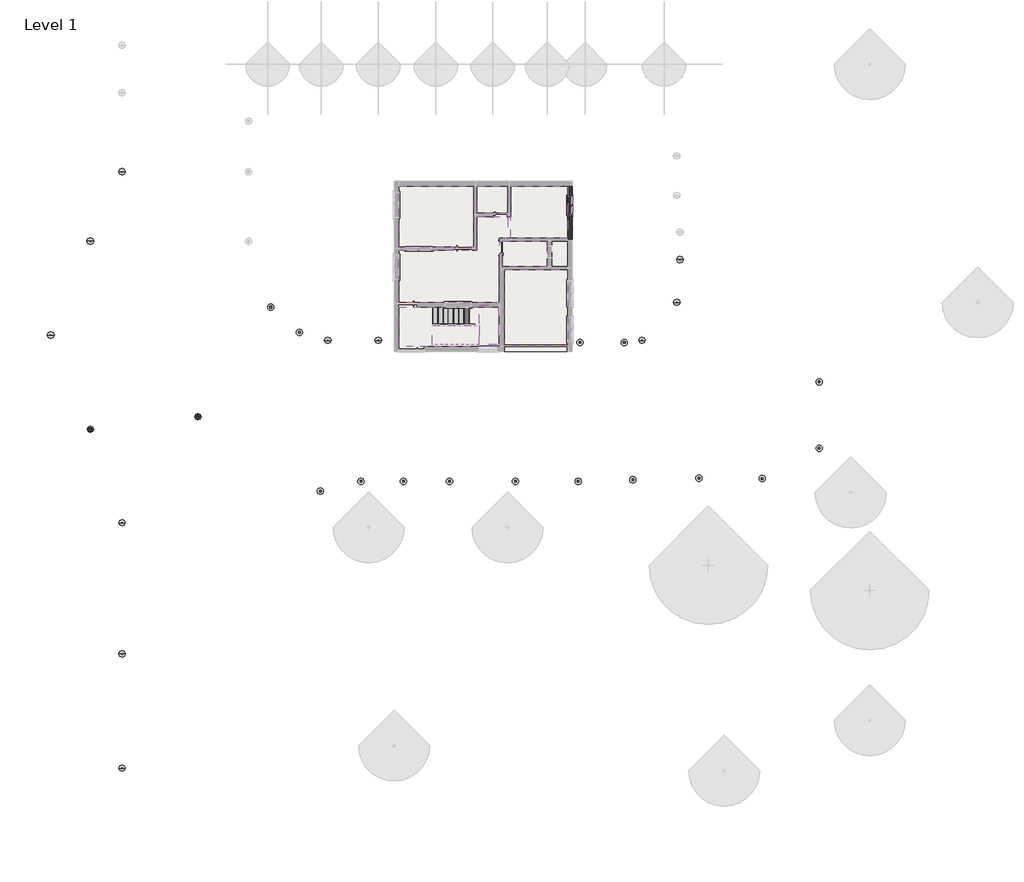
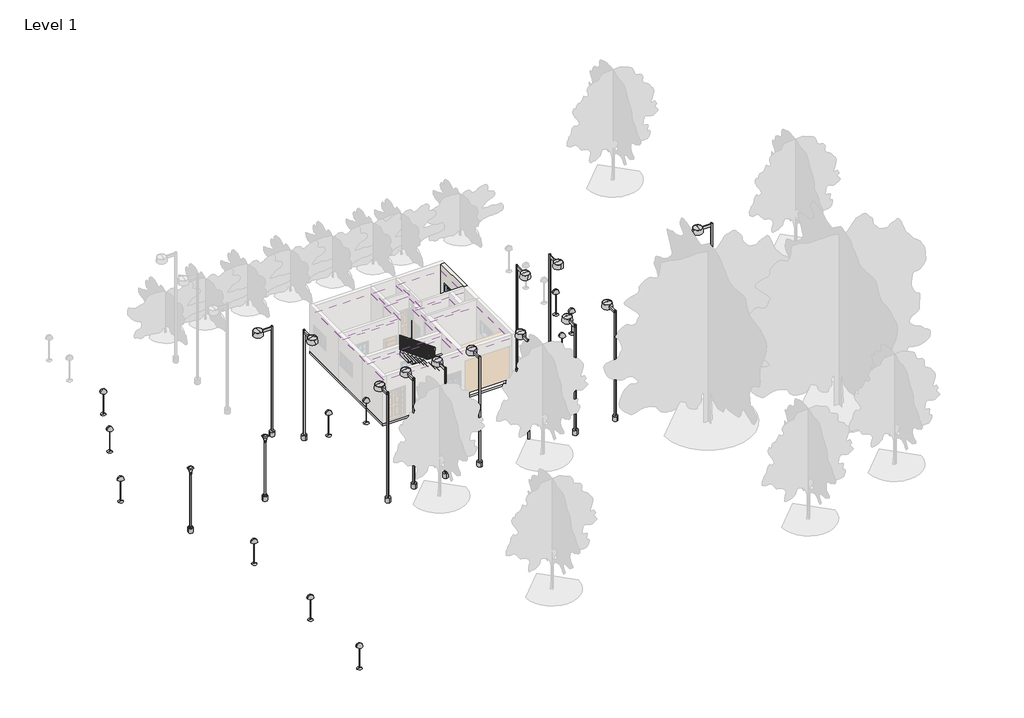
# One storey, part 2 of 3: 28 light fixtures, 7 coverings, 2 slabs, 2 stair flights, 1 railing, 1 wall, 1 window.
"""IFC4 building model written with IfcOpenShell, lengths in millimetres."""

from ifc_helpers import new_model, si_unit, frame, origin, place, context, project, spatial, polyline, outline, extrude, faceted_brep, transform, mapped, element, save
from components import m_floor_lamp_hemispheric_60w_120v_4a08ccbb, m_street_light_antique_400w_halogen_120v_ac89fb25, m_street_light_standard_250w_halogen_480v_204dbcbb, non_monolithic_landing_adbeca5e, stair_flight_50mm_tread_13mm_riser_with_nosing_6f61a695, stair_flight_50mm_tread_13mm_riser_with_nosing_ea10009b, m_window_casement_double_awning_double_3_6fa9dbfe

model = new_model("IFC4")

# Units and contexts
model_context = context("Model", 3, world=origin())
ifc_project = project(units=[si_unit("LENGTHUNIT", "METRE", prefix="MILLI")], contexts=[model_context])

# Site, building, storey
site = spatial("IfcSite", under=ifc_project)
building = spatial("IfcBuilding", under=site)
storey = spatial("IfcBuildingStorey", under=building, Name="Level 1", Elevation=0.0)

# Coverings
placement = place(None, origin())
element("IfcCovering", 1, ObjectType="Plain", at=placement, inside=storey, context=model_context, shape_type="SweptSolid", body=[
    extrude(outline(polyline([(-7823.0282945, 467.5578397), (-11429.8282945, 467.5578397), (-11429.8282945, 3413.9578397), (-7823.0282945, 3413.9578397), (-7823.0282945, 467.5578397)])), frame((0.0, 0.0, 2743.2), z_axis=(0.0, 0.0, 1.0), x_axis=(1.0, 0.0, 0.0)), (0.0, 0.0, 1.0), 57.0),
])
element("IfcCovering", 2, ObjectType="Plain", at=placement, inside=storey, context=model_context, shape_type="SweptSolid", body=[
    extrude(outline(polyline([(-7670.6282945, 2093.1578397), (-7670.6282945, 3413.9578397), (-6197.4282945, 3413.9578397), (-6197.4282945, 2093.1578397), (-7670.6282945, 2093.1578397)])), frame((0.0, 0.0, 2743.2), z_axis=(0.0, 0.0, 1.0), x_axis=(1.0, 0.0, 0.0)), (0.0, 0.0, 1.0), 57.0),
])
element("IfcCovering", 3, ObjectType="Plain", at=placement, inside=storey, context=model_context, shape_type="SweptSolid", body=[
    extrude(outline(polyline([(-11429.8282945, -2199.4421603), (-11429.8282945, 315.1578397), (-7670.6282945, 315.1578397), (-7670.6282945, 1940.7578397), (-6197.4282945, 1940.7578397), (-6197.4282945, 899.3578397), (-6603.8282945, 899.3578397), (-6603.8282945, -548.4421603), (-6603.8282945, -2199.4421603), (-11429.8282945, -2199.4421603)])), frame((0.0, 0.0, 2743.2), z_axis=(0.0, 0.0, 1.0), x_axis=(1.0, 0.0, 0.0)), (0.0, 0.0, 1.0), 57.0),
])
element("IfcCovering", 4, ObjectType="Plain", at=placement, inside=storey, context=model_context, shape_type="SweptSolid", body=[
    extrude(outline(polyline([(-6045.0282945, 899.3578397), (-6045.0282945, 3413.9578397), (-3301.8282945, 3413.9578397), (-3301.8282945, 899.3578397), (-6045.0282945, 899.3578397)])), frame((0.0, 0.0, 2743.2), z_axis=(0.0, 0.0, 1.0), x_axis=(1.0, 0.0, 0.0)), (0.0, 0.0, 1.0), 57.0),
])
element("IfcCovering", 5, ObjectType="Plain", at=placement, inside=storey, context=model_context, shape_type="SweptSolid", body=[
    extrude(outline(polyline([(-6451.4282945, 746.9578397), (-4292.4282945, 746.9578397), (-4292.4282945, -472.2421603), (-6451.4282945, -472.2421603), (-6451.4282945, 746.9578397)])), frame((0.0, 0.0, 2743.2), z_axis=(0.0, 0.0, 1.0), x_axis=(1.0, 0.0, 0.0)), (0.0, 0.0, 1.0), 57.0),
])
element("IfcCovering", 6, ObjectType="Plain", at=placement, inside=storey, context=model_context, shape_type="SweptSolid", body=[
    extrude(outline(polyline([(-6349.8282945, -624.6421603), (-3301.8282945, -624.6421603), (-3301.8282945, -4333.0421603), (-6349.8282945, -4333.0421603), (-6349.8282945, -624.6421603)])), frame((0.0, 0.0, 2743.2), z_axis=(0.0, 0.0, 1.0), x_axis=(1.0, 0.0, 0.0)), (0.0, 0.0, 1.0), 57.0),
])
element("IfcCovering", 7, ObjectType="Plain", at=placement, inside=storey, context=model_context, shape_type="SweptSolid", body=[
    extrude(outline(polyline([(-11429.8282945, -4333.0421603), (-11429.8282945, -2428.0421603), (-6603.8282945, -2428.0421603), (-6603.8282945, -4333.0421603), (-11429.8282945, -4333.0421603)])), frame((0.0, 0.0, 2743.2), z_axis=(0.0, 0.0, 1.0), x_axis=(1.0, 0.0, 0.0)), (0.0, 0.0, 1.0), 57.0),
])

# Light fixtures
m_floor_lamp_hemispheric_60w_120v_shape = m_floor_lamp_hemispheric_60w_120v_4a08ccbb(model_context)
element("IfcLightFixture", 8, ObjectType="M_Floor Lamp - Hemispheric : 60W - 120V", at=placement, inside=storey, context=model_context, shape_type="MappedRepresentation", body=[
    mapped(m_floor_lamp_hemispheric_60w_120v_shape, transform((-24764.8282945, 4099.7578397, 0.0), x_axis=(1.0, 0.0, 0.0), y_axis=(0.0, 1.0, 0.0), z_axis=(0.0, 0.0, 1.0))),
])
element("IfcLightFixture", 9, ObjectType="M_Floor Lamp - Hemispheric : 60W - 120V", at=placement, inside=storey, context=model_context, shape_type="MappedRepresentation", body=[
    mapped(m_floor_lamp_hemispheric_60w_120v_shape, transform((-26288.8282945, 746.9578397, 0.0), x_axis=(1.0, 0.0, 0.0), y_axis=(0.0, 1.0, 0.0), z_axis=(0.0, 0.0, 1.0))),
])
element("IfcLightFixture", 10, ObjectType="M_Floor Lamp - Hemispheric : 60W - 120V", at=placement, inside=storey, context=model_context, shape_type="MappedRepresentation", body=[
    mapped(m_floor_lamp_hemispheric_60w_120v_shape, transform((-28199.496103, -3776.7092743, 0.0), x_axis=(1.0, 0.0, 0.0), y_axis=(0.0, 1.0, 0.0), z_axis=(0.0, 0.0, 1.0))),
])
element("IfcLightFixture", 11, ObjectType="M_Floor Lamp - Hemispheric : 60W - 120V", at=placement, inside=storey, context=model_context, shape_type="MappedRepresentation", body=[
    mapped(m_floor_lamp_hemispheric_60w_120v_shape, transform((-24764.8282945, -12820.2421603, 0.0), x_axis=(1.0, 0.0, 0.0), y_axis=(0.0, 1.0, 0.0), z_axis=(0.0, 0.0, 1.0))),
])
element("IfcLightFixture", 12, ObjectType="M_Floor Lamp - Hemispheric : 60W - 120V", at=placement, inside=storey, context=model_context, shape_type="MappedRepresentation", body=[
    mapped(m_floor_lamp_hemispheric_60w_120v_shape, transform((-24764.8282945, -19145.2421603, 0.0), x_axis=(1.0, 0.0, 0.0), y_axis=(0.0, 1.0, 0.0), z_axis=(0.0, 0.0, 1.0))),
])
element("IfcLightFixture", 13, ObjectType="M_Floor Lamp - Hemispheric : 60W - 120V", at=placement, inside=storey, context=model_context, shape_type="MappedRepresentation", body=[
    mapped(m_floor_lamp_hemispheric_60w_120v_shape, transform((-24764.8282945, -24645.2421603, 0.0), x_axis=(1.0, 0.0, 0.0), y_axis=(0.0, 1.0, 0.0), z_axis=(0.0, 0.0, 1.0))),
])
element("IfcLightFixture", 14, ObjectType="M_Floor Lamp - Hemispheric : 60W - 120V", at=placement, inside=storey, context=model_context, shape_type="MappedRepresentation", body=[
    mapped(m_floor_lamp_hemispheric_60w_120v_shape, transform((2108.3717055, -142.0421603, 0.0), x_axis=(1.0, 0.0, 0.0), y_axis=(0.0, 1.0, 0.0), z_axis=(0.0, 0.0, 1.0))),
])
element("IfcLightFixture", 15, ObjectType="M_Floor Lamp - Hemispheric : 60W - 120V", at=placement, inside=storey, context=model_context, shape_type="MappedRepresentation", body=[
    mapped(m_floor_lamp_hemispheric_60w_120v_shape, transform((1955.9717055, -2199.4421603, 0.0), x_axis=(1.0, 0.0, 0.0), y_axis=(0.0, 1.0, 0.0), z_axis=(0.0, 0.0, 1.0))),
])
element("IfcLightFixture", 16, ObjectType="M_Floor Lamp - Hemispheric : 60W - 120V", at=placement, inside=storey, context=model_context, shape_type="MappedRepresentation", body=[
    mapped(m_floor_lamp_hemispheric_60w_120v_shape, transform((279.5717055, -4028.2421603, 0.0), x_axis=(1.0, 0.0, 0.0), y_axis=(0.0, 1.0, 0.0), z_axis=(0.0, 0.0, 1.0))),
])
element("IfcLightFixture", 17, ObjectType="M_Floor Lamp - Hemispheric : 60W - 120V", at=placement, inside=storey, context=model_context, shape_type="MappedRepresentation", body=[
    mapped(m_floor_lamp_hemispheric_60w_120v_shape, transform((-12420.4282945, -4028.2421603, 0.0), x_axis=(1.0, 0.0, 0.0), y_axis=(0.0, 1.0, 0.0), z_axis=(0.0, 0.0, 1.0))),
])
element("IfcLightFixture", 18, ObjectType="M_Floor Lamp - Hemispheric : 60W - 120V", at=placement, inside=storey, context=model_context, shape_type="MappedRepresentation", body=[
    mapped(m_floor_lamp_hemispheric_60w_120v_shape, transform((-14858.8282945, -4028.2421603, 0.0), x_axis=(1.0, 0.0, 0.0), y_axis=(0.0, 1.0, 0.0), z_axis=(0.0, 0.0, 1.0))),
])
m_street_light_antique_400w_halogen_120v_shape = m_street_light_antique_400w_halogen_120v_ac89fb25(model_context)
element("IfcLightFixture", 19, ObjectType="M_Street Light - Antique : 400W Halogen - 120V", at=placement, inside=storey, context=model_context, shape_type="MappedRepresentation", body=[
    mapped(m_street_light_antique_400w_halogen_120v_shape, transform((-21107.2282945, -7711.2421603, 0.0), x_axis=(1.0, 0.0, 0.0), y_axis=(0.0, 1.0, 0.0), z_axis=(0.0, 0.0, 1.0))),
])
element("IfcLightFixture", 20, ObjectType="M_Street Light - Antique : 400W Halogen - 120V", at=placement, inside=storey, context=model_context, shape_type="MappedRepresentation", body=[
    mapped(m_street_light_antique_400w_halogen_120v_shape, transform((-26288.8282945, -8320.8421603, 0.0), x_axis=(1.0, 0.0, 0.0), y_axis=(0.0, 1.0, 0.0), z_axis=(0.0, 0.0, 1.0))),
])
m_street_light_standard_250w_halogen_480v_shape = m_street_light_standard_250w_halogen_480v_204dbcbb(model_context)
element("IfcLightFixture", 21, ObjectType="M_Street Light - Standard : 250W Halogen - 480V", at=placement, inside=storey, context=model_context, shape_type="MappedRepresentation", body=[
    mapped(m_street_light_standard_250w_halogen_480v_shape, transform((-15213.0614004, -11296.4871366, 0.0), x_axis=(0.0, -1.0, 0.0), y_axis=(1.0, 0.0, 0.0), z_axis=(0.0, 0.0, 1.0))),
])
element("IfcLightFixture", 22, ObjectType="M_Street Light - Standard : 250W Halogen - 480V", at=placement, inside=storey, context=model_context, shape_type="MappedRepresentation", body=[
    mapped(m_street_light_standard_250w_halogen_480v_shape, transform((-13256.1020795, -10825.1754443, 0.0), x_axis=(0.0, -1.0, 0.0), y_axis=(1.0, 0.0, 0.0), z_axis=(0.0, 0.0, 1.0))),
])
element("IfcLightFixture", 23, ObjectType="M_Street Light - Standard : 250W Halogen - 480V", at=placement, inside=storey, context=model_context, shape_type="MappedRepresentation", body=[
    mapped(m_street_light_standard_250w_halogen_480v_shape, transform((-11210.6990221, -10825.1754443, 0.0), x_axis=(0.0, -1.0, 0.0), y_axis=(1.0, 0.0, 0.0), z_axis=(0.0, 0.0, 1.0))),
])
element("IfcLightFixture", 24, ObjectType="M_Street Light - Standard : 250W Halogen - 480V", at=placement, inside=storey, context=model_context, shape_type="MappedRepresentation", body=[
    mapped(m_street_light_standard_250w_halogen_480v_shape, transform((-8991.4282945, -10825.1754443, 0.0), x_axis=(0.0, -1.0, 0.0), y_axis=(1.0, 0.0, 0.0), z_axis=(0.0, 0.0, 1.0))),
])
element("IfcLightFixture", 25, ObjectType="M_Street Light - Standard : 250W Halogen - 480V", at=placement, inside=storey, context=model_context, shape_type="MappedRepresentation", body=[
    mapped(m_street_light_standard_250w_halogen_480v_shape, transform((-5816.409264, -10825.1754443, 0.0), x_axis=(0.0, -1.0, 0.0), y_axis=(1.0, 0.0, 0.0), z_axis=(0.0, 0.0, 1.0))),
])
element("IfcLightFixture", 26, ObjectType="M_Street Light - Standard : 250W Halogen - 480V", at=placement, inside=storey, context=model_context, shape_type="MappedRepresentation", body=[
    mapped(m_street_light_standard_250w_halogen_480v_shape, transform((-2793.8282945, -10825.1754443, 0.0), x_axis=(0.0, -1.0, 0.0), y_axis=(1.0, 0.0, 0.0), z_axis=(0.0, 0.0, 1.0))),
])
element("IfcLightFixture", 27, ObjectType="M_Street Light - Standard : 250W Halogen - 480V", at=placement, inside=storey, context=model_context, shape_type="MappedRepresentation", body=[
    mapped(m_street_light_standard_250w_halogen_480v_shape, transform((-160.8463909, -10748.9754443, 0.0), x_axis=(0.0, -1.0, 0.0), y_axis=(1.0, 0.0, 0.0), z_axis=(0.0, 0.0, 1.0))),
])
element("IfcLightFixture", 28, ObjectType="M_Street Light - Standard : 250W Halogen - 480V", at=placement, inside=storey, context=model_context, shape_type="MappedRepresentation", body=[
    mapped(m_street_light_standard_250w_halogen_480v_shape, transform((3022.7717055, -10672.7754443, 0.0), x_axis=(0.0, -1.0, 0.0), y_axis=(1.0, 0.0, 0.0), z_axis=(0.0, 0.0, 1.0))),
])
element("IfcLightFixture", 29, ObjectType="M_Street Light - Standard : 250W Halogen - 480V", at=placement, inside=storey, context=model_context, shape_type="MappedRepresentation", body=[
    mapped(m_street_light_standard_250w_halogen_480v_shape, transform((8813.9717055, -6034.8421603, 0.0), x_axis=(1.0, 0.0, 0.0), y_axis=(0.0, 1.0, 0.0), z_axis=(0.0, 0.0, 1.0))),
])
element("IfcLightFixture", 30, ObjectType="M_Street Light - Standard : 250W Halogen - 480V", at=placement, inside=storey, context=model_context, shape_type="MappedRepresentation", body=[
    mapped(m_street_light_standard_250w_halogen_480v_shape, transform((8813.9717055, -9235.2421603, 0.0), x_axis=(1.0, 0.0, 0.0), y_axis=(0.0, 1.0, 0.0), z_axis=(0.0, 0.0, 1.0))),
])
element("IfcLightFixture", 31, ObjectType="M_Street Light - Standard : 250W Halogen - 480V", at=placement, inside=storey, context=model_context, shape_type="MappedRepresentation", body=[
    mapped(m_street_light_standard_250w_halogen_480v_shape, transform((6070.7717055, -10690.9806356, 0.0), x_axis=(0.0, -1.0, 0.0), y_axis=(1.0, 0.0, 0.0), z_axis=(0.0, 0.0, 1.0))),
])
element("IfcLightFixture", 32, ObjectType="M_Street Light - Standard : 400W Halogen - 120V", at=placement, inside=storey, context=model_context, shape_type="MappedRepresentation", body=[
    mapped(m_street_light_standard_250w_halogen_480v_shape, transform((-17602.0282945, -2428.0421603, 0.0), x_axis=(1.0, 0.0, 0.0), y_axis=(0.0, 1.0, 0.0), z_axis=(0.0, 0.0, 1.0))),
])
element("IfcLightFixture", 33, ObjectType="M_Street Light - Standard : 400W Halogen - 120V", at=placement, inside=storey, context=model_context, shape_type="MappedRepresentation", body=[
    mapped(m_street_light_standard_250w_halogen_480v_shape, transform((-16221.6329612, -3647.2421603, 0.0), x_axis=(0.0, 1.0, 0.0), y_axis=(-1.0, 0.0, 0.0), z_axis=(0.0, 0.0, 1.0))),
])
element("IfcLightFixture", 34, ObjectType="M_Street Light - Standard : 400W Halogen - 120V", at=placement, inside=storey, context=model_context, shape_type="MappedRepresentation", body=[
    mapped(m_street_light_standard_250w_halogen_480v_shape, transform((-575.2329612, -4129.8421603, 0.0), x_axis=(0.0, 1.0, 0.0), y_axis=(-1.0, 0.0, 0.0), z_axis=(0.0, 0.0, 1.0))),
])
element("IfcLightFixture", 35, ObjectType="M_Street Light - Standard : 400W Halogen - 120V", at=placement, inside=storey, context=model_context, shape_type="MappedRepresentation", body=[
    mapped(m_street_light_standard_250w_halogen_480v_shape, transform((-2708.8329612, -4129.8421603, 0.0), x_axis=(0.0, 1.0, 0.0), y_axis=(-1.0, 0.0, 0.0), z_axis=(0.0, 0.0, 1.0))),
])

# Railing
element("IfcRailing", 36, ObjectType="1100mm", at=placement, inside=storey, context=model_context, shape_type="SolidModel", body=[
    faceted_brep([(-9804.2282945, -3247.1921603, 1277.8), (-9804.2282945, -3247.1921603, 1216.4443678), (-9804.2282945, -3297.1921603, 1216.4443678), (-9804.2282945, -3297.1921603, 1277.8), (-7604.2282945, -3247.1921603, 2842.44), (-7604.2282945, -3297.1921603, 2842.44), (-7604.2282945, -3297.1921603, 2781.0843678), (-7604.2282945, -3247.1921603, 2781.0843678)], [[[0, 1, 2, 3]], [[4, 5, 6, 7]], [[1, 0, 4, 7]], [[2, 1, 7, 6]], [[3, 2, 6, 5]], [[0, 3, 5, 4]]]),
    faceted_brep([(-7554.2282945, -3323.3921603, 3055.8), (-7604.2282945, -3323.3921603, 3030.0043678), (-7604.2282945, -3273.3921603, 3030.0043678), (-7554.2282945, -3273.3921603, 3055.8), (-9804.2282945, -3323.3921603, 4656.0), (-9804.2282945, -3273.3921603, 4656.0), (-9804.2282945, -3273.3921603, 4594.6443678), (-9804.2282945, -3323.3921603, 4594.6443678)], [[[0, 1, 2, 3]], [[4, 5, 6, 7]], [[1, 0, 4, 7]], [[2, 1, 7, 6]], [[3, 2, 6, 5]], [[0, 3, 5, 4]]]),
    faceted_brep([(-7554.2282945, -3247.1921603, 2878.0), (-7554.2282945, -3247.1921603, 2828.0), (-7604.2282945, -3247.1921603, 2828.0), (-7604.2282945, -3247.1921603, 2878.0), (-7554.2282945, -3273.3921603, 2878.0), (-7604.2282945, -3273.3921603, 2878.0), (-7604.2282945, -3323.3921603, 2828.0), (-7554.2282945, -3323.3921603, 2828.0)], [[[0, 1, 2, 3]], [[4, 5, 6, 7]], [[1, 0, 4, 7]], [[2, 1, 7, 6]], [[3, 2, 6, 5]], [[0, 3, 5, 4]]]),
    faceted_brep([(-7554.2282945, -3273.3921603, 2878.0), (-7554.2282945, -3323.3921603, 2828.0), (-7604.2282945, -3323.3921603, 2828.0), (-7604.2282945, -3273.3921603, 2878.0), (-7554.2282945, -3273.3921603, 3055.8), (-7604.2282945, -3273.3921603, 3030.0043678), (-7604.2282945, -3323.3921603, 3030.0043678), (-7554.2282945, -3323.3921603, 3055.8)], [[[0, 1, 2, 3]], [[4, 5, 6, 7]], [[1, 0, 4, 7]], [[2, 1, 7, 6]], [[3, 2, 6, 5]], [[0, 3, 5, 4]]]),
    extrude(outline(polyline([(3590.5281609, -9754.2282945), (4559.0843678, -9754.2282945), (4576.8643678, -9779.2282945), (3608.3081609, -9779.2282945), (3590.5281609, -9754.2282945)])), frame((0.0, -3310.8921603, 0.0), z_axis=(0.0, 1.0, 0.0), x_axis=(0.0, 0.0, 1.0)), (0.0, 0.0, 1.0), 25.0),
    extrude(outline(polyline([(3501.6281609, -9629.2282945), (4470.1843678, -9629.2282945), (4487.9643678, -9654.2282945), (3519.4081609, -9654.2282945), (3501.6281609, -9629.2282945)])), frame((0.0, -3310.8921603, 0.0), z_axis=(0.0, 1.0, 0.0), x_axis=(0.0, 0.0, 1.0)), (0.0, 0.0, 1.0), 25.0),
    extrude(outline(polyline([(3412.7281609, -9504.2282945), (4381.2843678, -9504.2282945), (4399.0643678, -9529.2282945), (3430.5081609, -9529.2282945), (3412.7281609, -9504.2282945)])), frame((0.0, -3310.8921603, 0.0), z_axis=(0.0, 1.0, 0.0), x_axis=(0.0, 0.0, 1.0)), (0.0, 0.0, 1.0), 25.0),
    extrude(outline(polyline([(3323.8281609, -9379.2282945), (4292.3843678, -9379.2282945), (4310.1643678, -9404.2282945), (3341.6081609, -9404.2282945), (3323.8281609, -9379.2282945)])), frame((0.0, -3310.8921603, 0.0), z_axis=(0.0, 1.0, 0.0), x_axis=(0.0, 0.0, 1.0)), (0.0, 0.0, 1.0), 25.0),
    extrude(outline(polyline([(3234.9281609, -9254.2282945), (4203.4843678, -9254.2282945), (4221.2643678, -9279.2282945), (3252.7081609, -9279.2282945), (3234.9281609, -9254.2282945)])), frame((0.0, -3310.8921603, 0.0), z_axis=(0.0, 1.0, 0.0), x_axis=(0.0, 0.0, 1.0)), (0.0, 0.0, 1.0), 25.0),
    extrude(outline(polyline([(3146.0281609, -9129.2282945), (4114.5843678, -9129.2282945), (4132.3643678, -9154.2282945), (3163.8081609, -9154.2282945), (3146.0281609, -9129.2282945)])), frame((0.0, -3310.8921603, 0.0), z_axis=(0.0, 1.0, 0.0), x_axis=(0.0, 0.0, 1.0)), (0.0, 0.0, 1.0), 25.0),
    extrude(outline(polyline([(3057.1281609, -9004.2282945), (4025.6843678, -9004.2282945), (4043.4643678, -9029.2282945), (3074.9081609, -9029.2282945), (3057.1281609, -9004.2282945)])), frame((0.0, -3310.8921603, 0.0), z_axis=(0.0, 1.0, 0.0), x_axis=(0.0, 0.0, 1.0)), (0.0, 0.0, 1.0), 25.0),
    extrude(outline(polyline([(2968.2281609, -8879.2282945), (3936.7843678, -8879.2282945), (3954.5643678, -8904.2282945), (2986.0081609, -8904.2282945), (2968.2281609, -8879.2282945)])), frame((0.0, -3310.8921603, 0.0), z_axis=(0.0, 1.0, 0.0), x_axis=(0.0, 0.0, 1.0)), (0.0, 0.0, 1.0), 25.0),
    extrude(outline(polyline([(2879.3281609, -8754.2282945), (3847.8843678, -8754.2282945), (3865.6643678, -8779.2282945), (2897.1081609, -8779.2282945), (2879.3281609, -8754.2282945)])), frame((0.0, -3310.8921603, 0.0), z_axis=(0.0, 1.0, 0.0), x_axis=(0.0, 0.0, 1.0)), (0.0, 0.0, 1.0), 25.0),
    extrude(outline(polyline([(2790.4281609, -8629.2282945), (3758.9843678, -8629.2282945), (3776.7643678, -8654.2282945), (2808.2081609, -8654.2282945), (2790.4281609, -8629.2282945)])), frame((0.0, -3310.8921603, 0.0), z_axis=(0.0, 1.0, 0.0), x_axis=(0.0, 0.0, 1.0)), (0.0, 0.0, 1.0), 25.0),
    extrude(outline(polyline([(2701.5281609, -8504.2282945), (3670.0843678, -8504.2282945), (3687.8643678, -8529.2282945), (2719.3081609, -8529.2282945), (2701.5281609, -8504.2282945)])), frame((0.0, -3310.8921603, 0.0), z_axis=(0.0, 1.0, 0.0), x_axis=(0.0, 0.0, 1.0)), (0.0, 0.0, 1.0), 25.0),
    extrude(outline(polyline([(2612.6281609, -8379.2282945), (3581.1843678, -8379.2282945), (3598.9643678, -8404.2282945), (2630.4081609, -8404.2282945), (2612.6281609, -8379.2282945)])), frame((0.0, -3310.8921603, 0.0), z_axis=(0.0, 1.0, 0.0), x_axis=(0.0, 0.0, 1.0)), (0.0, 0.0, 1.0), 25.0),
    extrude(outline(polyline([(2523.7281609, -8254.2282945), (3492.2843678, -8254.2282945), (3510.0643678, -8279.2282945), (2541.5081609, -8279.2282945), (2523.7281609, -8254.2282945)])), frame((0.0, -3310.8921603, 0.0), z_axis=(0.0, 1.0, 0.0), x_axis=(0.0, 0.0, 1.0)), (0.0, 0.0, 1.0), 25.0),
    extrude(outline(polyline([(2434.8281609, -8129.2282945), (3403.3843678, -8129.2282945), (3421.1643678, -8154.2282945), (2452.6081609, -8154.2282945), (2434.8281609, -8129.2282945)])), frame((0.0, -3310.8921603, 0.0), z_axis=(0.0, 1.0, 0.0), x_axis=(0.0, 0.0, 1.0)), (0.0, 0.0, 1.0), 25.0),
    extrude(outline(polyline([(2345.9281609, -8004.2282945), (3314.4843678, -8004.2282945), (3332.2643678, -8029.2282945), (2363.7081609, -8029.2282945), (2345.9281609, -8004.2282945)])), frame((0.0, -3310.8921603, 0.0), z_axis=(0.0, 1.0, 0.0), x_axis=(0.0, 0.0, 1.0)), (0.0, 0.0, 1.0), 25.0),
    extrude(outline(polyline([(2257.0281609, -7879.2282945), (3225.5843678, -7879.2282945), (3243.3643678, -7904.2282945), (2274.8081609, -7904.2282945), (2257.0281609, -7879.2282945)])), frame((0.0, -3310.8921603, 0.0), z_axis=(0.0, 1.0, 0.0), x_axis=(0.0, 0.0, 1.0)), (0.0, 0.0, 1.0), 25.0),
    extrude(outline(polyline([(2168.1281609, -7754.2282945), (3136.6843678, -7754.2282945), (3154.4643678, -7779.2282945), (2185.9081609, -7779.2282945), (2168.1281609, -7754.2282945)])), frame((0.0, -3310.8921603, 0.0), z_axis=(0.0, 1.0, 0.0), x_axis=(0.0, 0.0, 1.0)), (0.0, 0.0, 1.0), 25.0),
    extrude(outline(polyline([(2079.2281609, -7629.2282945), (3047.7843678, -7629.2282945), (3065.5643678, -7654.2282945), (2097.0081609, -7654.2282945), (2079.2281609, -7629.2282945)])), frame((0.0, -3310.8921603, 0.0), z_axis=(0.0, 1.0, 0.0), x_axis=(0.0, 0.0, 1.0)), (0.0, 0.0, 1.0), 25.0),
    extrude(outline(polyline([(2763.3043678, -7629.2282945), (1794.7481609, -7629.2282945), (1812.5281609, -7604.2282945), (2781.0843678, -7604.2282945), (2763.3043678, -7629.2282945)])), frame((0.0, -3284.6921603, 0.0), z_axis=(0.0, 1.0, 0.0), x_axis=(0.0, 0.0, 1.0)), (0.0, 0.0, 1.0), 25.0),
    extrude(outline(polyline([(2674.4043678, -7754.2282945), (1705.8481609, -7754.2282945), (1723.6281609, -7729.2282945), (2692.1843678, -7729.2282945), (2674.4043678, -7754.2282945)])), frame((0.0, -3284.6921603, 0.0), z_axis=(0.0, 1.0, 0.0), x_axis=(0.0, 0.0, 1.0)), (0.0, 0.0, 1.0), 25.0),
    extrude(outline(polyline([(2585.5043678, -7879.2282945), (1616.9481609, -7879.2282945), (1634.7281609, -7854.2282945), (2603.2843678, -7854.2282945), (2585.5043678, -7879.2282945)])), frame((0.0, -3284.6921603, 0.0), z_axis=(0.0, 1.0, 0.0), x_axis=(0.0, 0.0, 1.0)), (0.0, 0.0, 1.0), 25.0),
    extrude(outline(polyline([(2496.6043678, -8004.2282945), (1528.0481609, -8004.2282945), (1545.8281609, -7979.2282945), (2514.3843678, -7979.2282945), (2496.6043678, -8004.2282945)])), frame((0.0, -3284.6921603, 0.0), z_axis=(0.0, 1.0, 0.0), x_axis=(0.0, 0.0, 1.0)), (0.0, 0.0, 1.0), 25.0),
    extrude(outline(polyline([(2407.7043678, -8129.2282945), (1439.1481609, -8129.2282945), (1456.9281609, -8104.2282945), (2425.4843678, -8104.2282945), (2407.7043678, -8129.2282945)])), frame((0.0, -3284.6921603, 0.0), z_axis=(0.0, 1.0, 0.0), x_axis=(0.0, 0.0, 1.0)), (0.0, 0.0, 1.0), 25.0),
    extrude(outline(polyline([(2318.8043678, -8254.2282945), (1350.2481609, -8254.2282945), (1368.0281609, -8229.2282945), (2336.5843678, -8229.2282945), (2318.8043678, -8254.2282945)])), frame((0.0, -3284.6921603, 0.0), z_axis=(0.0, 1.0, 0.0), x_axis=(0.0, 0.0, 1.0)), (0.0, 0.0, 1.0), 25.0),
    extrude(outline(polyline([(2229.9043678, -8379.2282945), (1261.3481609, -8379.2282945), (1279.1281609, -8354.2282945), (2247.6843678, -8354.2282945), (2229.9043678, -8379.2282945)])), frame((0.0, -3284.6921603, 0.0), z_axis=(0.0, 1.0, 0.0), x_axis=(0.0, 0.0, 1.0)), (0.0, 0.0, 1.0), 25.0),
    extrude(outline(polyline([(2141.0043678, -8504.2282945), (1172.4481609, -8504.2282945), (1190.2281609, -8479.2282945), (2158.7843678, -8479.2282945), (2141.0043678, -8504.2282945)])), frame((0.0, -3284.6921603, 0.0), z_axis=(0.0, 1.0, 0.0), x_axis=(0.0, 0.0, 1.0)), (0.0, 0.0, 1.0), 25.0),
    extrude(outline(polyline([(2052.1043678, -8629.2282945), (1083.5481609, -8629.2282945), (1101.3281609, -8604.2282945), (2069.8843678, -8604.2282945), (2052.1043678, -8629.2282945)])), frame((0.0, -3284.6921603, 0.0), z_axis=(0.0, 1.0, 0.0), x_axis=(0.0, 0.0, 1.0)), (0.0, 0.0, 1.0), 25.0),
    extrude(outline(polyline([(1963.2043678, -8754.2282945), (994.6481609, -8754.2282945), (1012.4281609, -8729.2282945), (1980.9843678, -8729.2282945), (1963.2043678, -8754.2282945)])), frame((0.0, -3284.6921603, 0.0), z_axis=(0.0, 1.0, 0.0), x_axis=(0.0, 0.0, 1.0)), (0.0, 0.0, 1.0), 25.0),
    extrude(outline(polyline([(1874.3043678, -8879.2282945), (905.7481609, -8879.2282945), (923.5281609, -8854.2282945), (1892.0843678, -8854.2282945), (1874.3043678, -8879.2282945)])), frame((0.0, -3284.6921603, 0.0), z_axis=(0.0, 1.0, 0.0), x_axis=(0.0, 0.0, 1.0)), (0.0, 0.0, 1.0), 25.0),
    extrude(outline(polyline([(1785.4043678, -9004.2282945), (816.8481609, -9004.2282945), (834.6281609, -8979.2282945), (1803.1843678, -8979.2282945), (1785.4043678, -9004.2282945)])), frame((0.0, -3284.6921603, 0.0), z_axis=(0.0, 1.0, 0.0), x_axis=(0.0, 0.0, 1.0)), (0.0, 0.0, 1.0), 25.0),
    extrude(outline(polyline([(1696.5043678, -9129.2282945), (727.9481609, -9129.2282945), (745.7281609, -9104.2282945), (1714.2843678, -9104.2282945), (1696.5043678, -9129.2282945)])), frame((0.0, -3284.6921603, 0.0), z_axis=(0.0, 1.0, 0.0), x_axis=(0.0, 0.0, 1.0)), (0.0, 0.0, 1.0), 25.0),
    extrude(outline(polyline([(1607.6043678, -9254.2282945), (639.0481609, -9254.2282945), (656.8281609, -9229.2282945), (1625.3843678, -9229.2282945), (1607.6043678, -9254.2282945)])), frame((0.0, -3284.6921603, 0.0), z_axis=(0.0, 1.0, 0.0), x_axis=(0.0, 0.0, 1.0)), (0.0, 0.0, 1.0), 25.0),
    extrude(outline(polyline([(1518.7043678, -9379.2282945), (550.1481609, -9379.2282945), (567.9281609, -9354.2282945), (1536.4843678, -9354.2282945), (1518.7043678, -9379.2282945)])), frame((0.0, -3284.6921603, 0.0), z_axis=(0.0, 1.0, 0.0), x_axis=(0.0, 0.0, 1.0)), (0.0, 0.0, 1.0), 25.0),
    extrude(outline(polyline([(1429.8043678, -9504.2282945), (461.2481609, -9504.2282945), (479.0281609, -9479.2282945), (1447.5843678, -9479.2282945), (1429.8043678, -9504.2282945)])), frame((0.0, -3284.6921603, 0.0), z_axis=(0.0, 1.0, 0.0), x_axis=(0.0, 0.0, 1.0)), (0.0, 0.0, 1.0), 25.0),
    extrude(outline(polyline([(1340.9043678, -9629.2282945), (372.3481609, -9629.2282945), (390.1281609, -9604.2282945), (1358.6843678, -9604.2282945), (1340.9043678, -9629.2282945)])), frame((0.0, -3284.6921603, 0.0), z_axis=(0.0, 1.0, 0.0), x_axis=(0.0, 0.0, 1.0)), (0.0, 0.0, 1.0), 25.0),
    extrude(outline(polyline([(1252.0043678, -9754.2282945), (283.4481609, -9754.2282945), (301.2281609, -9729.2282945), (1269.7843678, -9729.2282945), (1252.0043678, -9754.2282945)])), frame((0.0, -3284.6921603, 0.0), z_axis=(0.0, 1.0, 0.0), x_axis=(0.0, 0.0, 1.0)), (0.0, 0.0, 1.0), 25.0),
    extrude(outline(polyline([(-3285.8921603, 2828.0), (-3285.8921603, 2034.7781609), (-3310.8921603, 2052.5581609), (-3310.8921603, 2828.0), (-3285.8921603, 2828.0)])), frame((-7591.7282945, 0.0, 0.0), z_axis=(1.0, 0.0, 0.0), x_axis=(0.0, 1.0, 0.0)), (0.0, 0.0, 1.0), 25.0),
    extrude(outline(polyline([(2789.9743678, -7591.7282945), (1828.0, -7591.7282945), (1828.0, -7566.7282945), (2807.7543678, -7566.7282945), (2789.9743678, -7591.7282945)])), frame((0.0, -3284.6921603, 0.0), z_axis=(0.0, 1.0, 0.0), x_axis=(0.0, 0.0, 1.0)), (0.0, 0.0, 1.0), 25.0),
    extrude(outline(polyline([(3608.3081609, -9779.2282945), (4576.8643678, -9779.2282945), (4594.6443678, -9804.2282945), (3626.0881609, -9804.2282945), (3608.3081609, -9779.2282945)])), frame((0.0, -3310.8921603, 0.0), z_axis=(0.0, 1.0, 0.0), x_axis=(0.0, 0.0, 1.0)), (0.0, 0.0, 1.0), 25.0),
    extrude(outline(polyline([(1216.4443678, -9804.2282945), (247.8881609, -9804.2282945), (265.6681609, -9779.2282945), (1234.2243678, -9779.2282945), (1216.4443678, -9804.2282945)])), frame((0.0, -3284.6921603, 0.0), z_axis=(0.0, 1.0, 0.0), x_axis=(0.0, 0.0, 1.0)), (0.0, 0.0, 1.0), 25.0),
])

# Slabs
element("IfcSlab", 37, ObjectType="Generic 150mm", at=placement, inside=storey, context=model_context, shape_type="SweptSolid", body=[
    extrude(outline(polyline([(-11658.4282945, -4561.6421603), (-11658.4282945, 3642.5578397), (-3073.2282945, 3642.5578397), (-3073.2282945, -4561.6421603), (-11658.4282945, -4561.6421603)])), frame((0.0, 0.0, -150.0), z_axis=(0.0, 0.0, 1.0), x_axis=(1.0, 0.0, 0.0)), (0.0, 0.0, 1.0), 150.0),
])
non_monolithic_landing_shape = non_monolithic_landing_adbeca5e(model_context)
element("IfcSlab", 38, ObjectType="Non-Monolithic Landing", at=placement, inside=storey, context=model_context, shape_type="MappedRepresentation", body=[
    mapped(non_monolithic_landing_shape, transform((0.0, 0.0, 0.0), x_axis=(1.0, 0.0, 0.0), y_axis=(0.0, 1.0, 0.0), z_axis=(0.0, 0.0, 1.0))),
])

# Stair flights
stair_flight_50mm_tread_13mm_riser_with_nosing_shape = stair_flight_50mm_tread_13mm_riser_with_nosing_6f61a695(model_context)
element("IfcStairFlight", 39, ObjectType="50mm Tread 13mm Riser with Nosing", at=placement, inside=storey, context=model_context, shape_type="MappedRepresentation", body=[
    mapped(stair_flight_50mm_tread_13mm_riser_with_nosing_shape, transform((0.0, 0.0, 0.0), x_axis=(1.0, 0.0, 0.0), y_axis=(0.0, 1.0, 0.0), z_axis=(0.0, 0.0, 1.0))),
])
stair_flight_50mm_tread_13mm_riser_with_nosing_2_shape = stair_flight_50mm_tread_13mm_riser_with_nosing_ea10009b(model_context)
element("IfcStairFlight", 40, ObjectType="50mm Tread 13mm Riser with Nosing", at=placement, inside=storey, context=model_context, shape_type="MappedRepresentation", body=[
    mapped(stair_flight_50mm_tread_13mm_riser_with_nosing_2_shape, transform((0.0, 0.0, 0.0), x_axis=(1.0, 0.0, 0.0), y_axis=(0.0, 1.0, 0.0), z_axis=(0.0, 0.0, 1.0))),
])

# Wall
element("IfcWall", 41, ObjectType="9\"", at=placement, inside=storey, context=model_context, shape_type="Brep", body=[
    faceted_brep([(-3301.8282945, 3413.9578397, 0.0), (-3301.8282945, 899.3578397, 0.0), (-3301.8282945, 823.1578397, 0.0), (-3301.8282945, 823.1578397, 3200.4), (-3301.8282945, 899.3578397, 3200.4), (-3301.8282945, 3413.9578397, 3200.4), (-3301.8282945, 2016.9578397, 2119.2), (-3301.8282945, 2016.9578397, 1219.2), (-3301.8282945, 2931.3578397, 1219.2), (-3301.8282945, 2931.3578397, 2119.2), (-3073.2282945, 3413.9578397, 0.0), (-3073.2282945, 3413.9578397, 3200.4), (-3073.2282945, 823.1578397, 3200.4), (-3073.2282945, 823.1578397, 0.0), (-3073.2282945, 2016.9578397, 2119.2), (-3073.2282945, 2931.3578397, 2119.2), (-3073.2282945, 2931.3578397, 1219.2), (-3073.2282945, 2016.9578397, 1219.2)], [[[0, 1, 2, 3, 4, 5], [6, 7, 8, 9]], [[10, 11, 12, 13], [14, 15, 16, 17]], [[2, 1, 0, 10, 13]], [[3, 2, 13, 12]], [[5, 4, 3, 12, 11]], [[0, 5, 11, 10]], [[7, 6, 14, 17]], [[8, 7, 17, 16]], [[9, 8, 16, 15]], [[6, 9, 15, 14]]]),
])

# Window
m_window_casement_double_awning_double_3_shape = m_window_casement_double_awning_double_3_6fa9dbfe(model_context)
element("IfcWindow", 42, ObjectType="M_Window-Casement-Double-Awning-Double : 3'", at=placement, inside=storey, context=model_context, shape_type="MappedRepresentation", body=[
    mapped(m_window_casement_double_awning_double_3_shape, transform((-3187.5282945, 2474.1578397, 319.2), x_axis=(0.0, -1.0, 0.0), y_axis=(1.0, 0.0, 0.0), z_axis=(0.0, 0.0, 1.0))),
])

save(model, "model.ifc")

# Revit data of these elements
# Type "Plain"
#   built-in parameter 1002203 = 1 (stored number, unit not read)
#   built-in parameter 1002202 = 1 (stored number, unit not read)
#   Layers, outside or top first: 0' - 1.77165" "Metal Stud Layer" (function 1); 0' - 0.47244" "Gypsum Wall Board" (function 1)
# Type "M_Floor Lamp - Hemispheric : 60W - 120V"
#   Photometric Web File = "CLFR1A19.ies"
#   Assembly Code = "D5020220"
#   Lamp = "A-19"
#   Wattage Comments = "60"
#   Wattage = 500 W
#   built-in parameter 1150110 = 2 (stored number, unit not read)
#   built-in parameter 1114217 = 4 (stored number, unit not read)
#   built-in parameter 1150109 = 2 (stored number, unit not read)
#   built-in parameter 1150113 = 1 (stored number, unit not read)
#   Tilt Angle = 90.00°
#   built-in parameter 1150115 = 1 (stored number, unit not read)
#   built-in parameter 1150105 = 3988.82 (stored number, unit not read)
#   built-in parameter 1150112 = 1 (stored number, unit not read)
#   built-in parameter 1150114 = 1 (stored number, unit not read)
#   built-in parameter 1150107 = 6500 (stored number, unit not read)
#   built-in parameter 1150106 = 39.8882 (stored number, unit not read)
#   built-in parameter 1150104 = 9.31353 (stored number, unit not read)
#   Ballast Voltage = 120 V
#   built-in parameter 1114218 = 1 (stored number, unit not read)
#   built-in parameter 1150133 = 10 (stored number, unit not read)
#   Lumens = 50125 lm
#   Apparent Load = 60 VA
#   built-in parameter 1150134 = 1
#   built-in parameter 1150137 = 1
#   Color Filter = 16777215
#   Ballast Number of Poles = 1
#   Stand = Steel, Chrome Plated
#   Shade = Glass, Frosted
#   Dimming Lamp Color Temperature Shift = (empty or 0)
#   Default Elevation = 0
# Type "M_Street Light - Antique : 400W Halogen - 120V"
#   Photometric Web File = "SLS1T3.ies"
#   Assembly Code = "D5020280"
#   Lamp = "T-3"
#   Wattage Comments = "400"
#   Wattage = 1000 W
#   built-in parameter 1150110 = 2 (stored number, unit not read)
#   built-in parameter 1114217 = 4 (stored number, unit not read)
#   built-in parameter 1150109 = 2 (stored number, unit not read)
#   built-in parameter 1150113 = 1 (stored number, unit not read)
#   Tilt Angle = -90.00°
#   built-in parameter 1150115 = 1 (stored number, unit not read)
#   built-in parameter 1150105 = 7957.75 (stored number, unit not read)
#   built-in parameter 1150112 = 1 (stored number, unit not read)
#   built-in parameter 1150114 = 1 (stored number, unit not read)
#   built-in parameter 1150107 = 8000 (stored number, unit not read)
#   built-in parameter 1150106 = 79.5775 (stored number, unit not read)
#   built-in parameter 1150104 = 9.2903 (stored number, unit not read)
#   Voltage = 120 V
#   built-in parameter 1114218 = 1 (stored number, unit not read)
#   built-in parameter 1150133 = 10 (stored number, unit not read)
#   Height = 14' - 9.16535"
#   Lumens = 100000 lm
#   Apparent Load = 400 VA
#   built-in parameter 1150137 = 1
#   Color Filter = 16777215
#   Number of poles = 1
#   Shade Material = none
#   Load Classification = Lighting - Exterior
#   Diffuser Material = Glass, Frosted
#   Stand Material = Steel, Paint Finish, Dark Gray, Matte
#   Dimming Lamp Color Temperature Shift = (empty or 0)
#   Default Elevation = 0
# Type "M_Street Light - Standard : 250W Halogen - 480V"
#   Photometric Web File = "SLS1T4.IES"
#   Lamp = "T-4"
#   Wattage Comments = "250"
#   Wattage = 1000 W
#   built-in parameter 1150110 = 2 (stored number, unit not read)
#   built-in parameter 1114217 = 4 (stored number, unit not read)
#   built-in parameter 1150109 = 2 (stored number, unit not read)
#   built-in parameter 1150113 = 1 (stored number, unit not read)
#   Tilt Angle = -90.00°
#   built-in parameter 1150115 = 1 (stored number, unit not read)
#   built-in parameter 1150105 = 7957.75 (stored number, unit not read)
#   built-in parameter 1150112 = 1 (stored number, unit not read)
#   built-in parameter 1150114 = 1 (stored number, unit not read)
#   built-in parameter 1150107 = 6500 (stored number, unit not read)
#   built-in parameter 1150106 = 79.5775 (stored number, unit not read)
#   Height = 24' - 7.27559"
#   Lumens = 100000 lm
#   built-in parameter 1150104 = 9.2903 (stored number, unit not read)
#   Voltage = 480 V
#   built-in parameter 1114218 = 1 (stored number, unit not read)
#   built-in parameter 1150133 = 10 (stored number, unit not read)
#   Apparent Load = 250 VA
#   built-in parameter 1150134 = 1
#   built-in parameter 1150137 = 1
#   Color Filter = 16777215
#   Number of poles = 3
#   Stand Material = Steel, Paint Finish, Dark Gray, Matte
#   Shade Material = Steel, Paint Finish, Dark Gray, Matte
#   Load Classification = Lighting - Exterior
#   Diffuser Material = Glass, Frosted
#   Dimming Lamp Color Temperature Shift = (empty or 0)
#   Default Elevation = 0
# Type "M_Street Light - Standard : 400W Halogen - 120V"
#   Photometric Web File = "SLS1T3.ies"
#   Lamp = "T-3"
#   Wattage Comments = "400"
#   Wattage = 1000 W
#   built-in parameter 1150110 = 2 (stored number, unit not read)
#   built-in parameter 1114217 = 4 (stored number, unit not read)
#   built-in parameter 1150109 = 2 (stored number, unit not read)
#   built-in parameter 1150113 = 1 (stored number, unit not read)
#   Tilt Angle = -90.00°
#   built-in parameter 1150115 = 1 (stored number, unit not read)
#   built-in parameter 1150105 = 7957.75 (stored number, unit not read)
#   built-in parameter 1150112 = 1 (stored number, unit not read)
#   built-in parameter 1150114 = 1 (stored number, unit not read)
#   built-in parameter 1150107 = 6500 (stored number, unit not read)
#   built-in parameter 1150106 = 79.5775 (stored number, unit not read)
#   Height = 24' - 7.27559"
#   Lumens = 100000 lm
#   built-in parameter 1150104 = 9.2903 (stored number, unit not read)
#   Voltage = 120 V
#   built-in parameter 1114218 = 1 (stored number, unit not read)
#   built-in parameter 1150133 = 10 (stored number, unit not read)
#   Apparent Load = 400 VA
#   built-in parameter 1150134 = 1
#   built-in parameter 1150137 = 1
#   Color Filter = 16777215
#   Number of poles = 1
#   Stand Material = Steel, Paint Finish, Dark Gray, Matte
#   Shade Material = Steel, Paint Finish, Dark Gray, Matte
#   Load Classification = Lighting - Exterior
#   Diffuser Material = Glass, Frosted
#   Dimming Lamp Color Temperature Shift = (empty or 0)
#   Default Elevation = 0
# Type "1100mm"
#   built-in parameter 1008612 = 0.019685 (stored number, unit not read)
#   built-in parameter 1008611 = 0.019685 (stored number, unit not read)
#   built-in parameter 1008609 = 0.902231 (stored number, unit not read)
#   built-in parameter 1008604 = 0.19685 (stored number, unit not read)
#   built-in parameter 1008603 = 0.164042 (stored number, unit not read)
#   Railing Height = 3' - 7.30709"
#   built-in parameter 1008630 = 2
#   built-in parameter 1008610 = 2
#   built-in parameter 1008608 = 1
#   built-in parameter 1008618 = M_Baluster - Square : 25mm
# Type "Generic 150mm"
#   Function = 0
#   Layers, outside or top first: 0' - 5.90551" no material (function 1)
# Type "9\""
#   Layers, outside or top first: 0' - 9" no material (function 1)
# Type "M_Window-Casement-Double-Awning-Double : 3'"
#   Type Mark = "31"
#   Fire Rating = "0.5h"
#   Assembly Code = "B2020100"
#   Analytic Construction = "Double glazing - domestic"
#   Window Inset [instance default] = 0' - 0"
#   Wall Thickness [instance default] = 0' - 5.90551"
#   Interior Wall Closure [instance default] = 0' - 2.15551"
#   Half Width = 1' - 6"
#   Visual Light Transmittance = 0.81
#   Transom Height = 0' - 11.81102"
#   Thermal Resistance (R) = 0.319569 (m²·K)/W
#   Solar Heat Gain Coefficient = 0.76
#   Rough Width = 3' - 0.59055"
#   Rough Height = 3' - 0.02362"
#   Open Window Height = 1' - 11.62205"
#   Frame Extension [instance default] = 0' - 0 1/4"
#   Height = 2' - 11.43307"
#   Heat Transfer Coefficient (U) = 3.12929 W/(m²·K)
#   Exterior Wall Closure [instance default] = 0' - 1.25197"
#   Extension Jamb [instance default] = 0' - 2.15551"
#   Default Sill Height = 2' - 11.43307"
#   Width = 3' - 0"
#   Top Muntin Visibility = yes
#   Bottom Muntin Visibility = yes
#   Interior Trim Visibility [instance default] = yes
#   Exterior Trim Visibility [instance default] = yes
#   Extension Jamb Visibility [instance default] = yes
#   Interior Trim Material = Wood - Stained
#   Muntin Pattern = M_Muntin Pattern_2x2 : M_Muntin Pattern_2x2
#   Interior Trim = M_Trim-Window-Interior-Flat : Picture Frame
#   Interior Frame Material = Wood - Stained
#   Glass Panel Material = Glass
#   Exterior Trim Material = Clad - White
#   Exterior Trim = M_Trim-Window-Exterior-Flat : with Sill
#   Exterior Frame Material = Clad - White
#   Wall Closure = (empty or 0)
# Elements 1, 2, 3, 4, 5, 6, 7 (IfcCovering, "Plain")
#   Height Offset From Level = 9' - 0"
#   Phase Created = New Construction
#   Materials on its faces: "Gypsum Wall Board", "Metal Stud Layer"
# Element 8 (IfcLightFixture, "M_Floor Lamp - Hemispheric : 60W - 120V")
#   Mark = "10"
#   Phase Created = New Construction
#   Materials on its faces: "Steel, Chrome Plated", "Glass, Frosted"
# Element 9 (IfcLightFixture, "M_Floor Lamp - Hemispheric : 60W - 120V")
#   Mark = "11"
#   Phase Created = New Construction
#   Materials on its faces: "Steel, Chrome Plated", "Glass, Frosted"
# Element 10 (IfcLightFixture, "M_Floor Lamp - Hemispheric : 60W - 120V")
#   Mark = "12"
#   Phase Created = New Construction
#   Materials on its faces: "Steel, Chrome Plated", "Glass, Frosted"
# Element 11 (IfcLightFixture, "M_Floor Lamp - Hemispheric : 60W - 120V")
#   Mark = "13"
#   Phase Created = New Construction
#   Materials on its faces: "Steel, Chrome Plated", "Glass, Frosted"
# Element 12 (IfcLightFixture, "M_Floor Lamp - Hemispheric : 60W - 120V")
#   Mark = "14"
#   Phase Created = New Construction
#   Materials on its faces: "Steel, Chrome Plated", "Glass, Frosted"
# Element 13 (IfcLightFixture, "M_Floor Lamp - Hemispheric : 60W - 120V")
#   Mark = "15"
#   Phase Created = New Construction
#   Materials on its faces: "Steel, Chrome Plated", "Glass, Frosted"
# Element 14 (IfcLightFixture, "M_Floor Lamp - Hemispheric : 60W - 120V")
#   Mark = "19"
#   Phase Created = New Construction
#   Materials on its faces: "Steel, Chrome Plated", "Glass, Frosted"
# Element 15 (IfcLightFixture, "M_Floor Lamp - Hemispheric : 60W - 120V")
#   Mark = "20"
#   Phase Created = New Construction
#   Materials on its faces: "Steel, Chrome Plated", "Glass, Frosted"
# Element 16 (IfcLightFixture, "M_Floor Lamp - Hemispheric : 60W - 120V")
#   Mark = "21"
#   Phase Created = New Construction
#   Materials on its faces: "Steel, Chrome Plated", "Glass, Frosted"
# Element 17 (IfcLightFixture, "M_Floor Lamp - Hemispheric : 60W - 120V")
#   Mark = "22"
#   Phase Created = New Construction
#   Materials on its faces: "Steel, Chrome Plated", "Glass, Frosted"
# Element 18 (IfcLightFixture, "M_Floor Lamp - Hemispheric : 60W - 120V")
#   Mark = "23"
#   Phase Created = New Construction
#   Materials on its faces: "Steel, Chrome Plated", "Glass, Frosted"
# Element 19 (IfcLightFixture, "M_Street Light - Antique : 400W Halogen - 120V")
#   Mark = "25"
#   Phase Created = New Construction
#   Materials on its faces: "Steel, Paint Finish, Dark Gray, Matte", "Glass, Frosted"
# Element 20 (IfcLightFixture, "M_Street Light - Antique : 400W Halogen - 120V")
#   Mark = "26"
#   Phase Created = New Construction
#   Materials on its faces: "Steel, Paint Finish, Dark Gray, Matte", "Glass, Frosted"
# Element 21 (IfcLightFixture, "M_Street Light - Standard : 250W Halogen - 480V")
#   Mark = "27"
#   Phase Created = New Construction
#   Materials on its faces: "Steel, Paint Finish, Dark Gray, Matte", "Glass, Frosted"
# Element 22 (IfcLightFixture, "M_Street Light - Standard : 250W Halogen - 480V")
#   Mark = "28"
#   Phase Created = New Construction
#   Materials on its faces: "Steel, Paint Finish, Dark Gray, Matte", "Glass, Frosted"
# Element 23 (IfcLightFixture, "M_Street Light - Standard : 250W Halogen - 480V")
#   Mark = "29"
#   Phase Created = New Construction
#   Materials on its faces: "Steel, Paint Finish, Dark Gray, Matte", "Glass, Frosted"
# Element 24 (IfcLightFixture, "M_Street Light - Standard : 250W Halogen - 480V")
#   Mark = "30"
#   Phase Created = New Construction
#   Materials on its faces: "Steel, Paint Finish, Dark Gray, Matte", "Glass, Frosted"
# Element 25 (IfcLightFixture, "M_Street Light - Standard : 250W Halogen - 480V")
#   Mark = "31"
#   Phase Created = New Construction
#   Materials on its faces: "Steel, Paint Finish, Dark Gray, Matte", "Glass, Frosted"
# Element 26 (IfcLightFixture, "M_Street Light - Standard : 250W Halogen - 480V")
#   Mark = "32"
#   Phase Created = New Construction
#   Materials on its faces: "Steel, Paint Finish, Dark Gray, Matte", "Glass, Frosted"
# Element 27 (IfcLightFixture, "M_Street Light - Standard : 250W Halogen - 480V")
#   Mark = "33"
#   Phase Created = New Construction
#   Materials on its faces: "Steel, Paint Finish, Dark Gray, Matte", "Glass, Frosted"
# Element 28 (IfcLightFixture, "M_Street Light - Standard : 250W Halogen - 480V")
#   Mark = "34"
#   Phase Created = New Construction
#   Materials on its faces: "Steel, Paint Finish, Dark Gray, Matte", "Glass, Frosted"
# Element 29 (IfcLightFixture, "M_Street Light - Standard : 250W Halogen - 480V")
#   Mark = "35"
#   Phase Created = New Construction
#   Materials on its faces: "Steel, Paint Finish, Dark Gray, Matte", "Glass, Frosted"
# Element 30 (IfcLightFixture, "M_Street Light - Standard : 250W Halogen - 480V")
#   Mark = "36"
#   Phase Created = New Construction
#   Materials on its faces: "Steel, Paint Finish, Dark Gray, Matte", "Glass, Frosted"
# Element 31 (IfcLightFixture, "M_Street Light - Standard : 250W Halogen - 480V")
#   Mark = "37"
#   Phase Created = New Construction
#   Materials on its faces: "Steel, Paint Finish, Dark Gray, Matte", "Glass, Frosted"
# Element 32 (IfcLightFixture, "M_Street Light - Standard : 400W Halogen - 120V")
#   Mark = "4"
#   Phase Created = New Construction
#   Materials on its faces: "Steel, Paint Finish, Dark Gray, Matte", "Glass, Frosted"
# Element 33 (IfcLightFixture, "M_Street Light - Standard : 400W Halogen - 120V")
#   Mark = "5"
#   Phase Created = New Construction
#   Materials on its faces: "Steel, Paint Finish, Dark Gray, Matte", "Glass, Frosted"
# Element 34 (IfcLightFixture, "M_Street Light - Standard : 400W Halogen - 120V")
#   Mark = "6"
#   Phase Created = New Construction
#   Materials on its faces: "Steel, Paint Finish, Dark Gray, Matte", "Glass, Frosted"
# Element 35 (IfcLightFixture, "M_Street Light - Standard : 400W Halogen - 120V")
#   Mark = "7"
#   Phase Created = New Construction
#   Materials on its faces: "Steel, Paint Finish, Dark Gray, Matte", "Glass, Frosted"
# Element 36 (IfcRailing, "1100mm")
#   Phase Created = New Construction
# Element 37 (IfcSlab, "Generic 150mm")
#   built-in parameter 1001955 = -1.5708 (stored number, unit not read)
#   Height Offset From Level = 0' - 0"
#   Phase Created = New Construction
#   Materials on its faces: "Default Floor", "FLOORING TILES"
# Element 38 (IfcSlab, "Non-Monolithic Landing")
#   Phase Created = New Construction
# Elements 39, 40 (IfcStairFlight, "50mm Tread 13mm Riser with Nosing")
#   Phase Created = New Construction
# Element 41 (IfcWall, "9\"")
#   Top Offset = 0' - 0"
#   Base Offset = 0' - 0"
#   Unconnected Height = 10' - 6"
#   wall height = 10' - 6"
#   Phase Created = New Construction
#   Base Constraint = Level 1
#   Materials on its faces: "Default Wall", "LIVING ROOM WALL2", "OUTER WALL"
# Element 42 (IfcWindow, "M_Window-Casement-Double-Awning-Double : 3'")
#   Mark = "8"
#   Window Inset = 0' - 0"
#   Interior Wall Closure = 0' - 2.15551"
#   Frame Extension = 0' - 0 1/4"
#   Exterior Wall Closure = 0' - 1.25197"
#   Interior Trim Visibility = yes
#   Exterior Trim Visibility = yes
#   Phase Created = New Construction
#   Materials on its faces: "Wood - Stained", "Glass", "Clad - White"
# Materials
#   "Metal Stud Layer": class "Metal", colour RGB 127 127 127, transparency 0, Description = "Light gauge steel framing, thermal air layer", Cost = 0
#   "Gypsum Wall Board": class "Generic", colour RGB 249 249 249, transparency 0, Description = "Gypsum Wall Board", Cost = 0
#   "Steel, Chrome Plated": class "Metal", colour RGB 17 17 17, transparency 0, Description = "Chromiuim plated steel", Cost = 0
#   "Glass, Frosted": class "Glass", colour RGB 249 250 249, transparency 0.8, Description = "physical material", Cost = 0
#   "Steel, Paint Finish, Dark Gray, Matte": class "Metal", colour RGB 98 98 98, transparency 0, Description = "Steel, paint finish, dark gray, matte", Cost = 0
#   "Wood - Stained": class "Wood", colour RGB 224 178 126, transparency 0, Cost = 0
#   "Glass": class "Glass", colour RGB 0 128 192, transparency 0.9, Description = "Soda Lime Glass", Cost = 0
#   "Clad - White": class "Wood", colour RGB 242 242 238, transparency 0, Cost = 0
#   "Default Floor": colour RGB 127 127 127, transparency 0, Cost = 0
#   "FLOORING TILES": class "Generic", colour RGB 120 120 120, transparency 0, Cost = 0
#   "Default Wall": colour RGB 128 128 128, transparency 0, Cost = 0
#   "LIVING ROOM WALL2": class "Generic", colour RGB 120 120 120, transparency 0, Cost = 0
#   "OUTER WALL": class "Generic", colour RGB 120 120 120, transparency 0, Cost = 0
